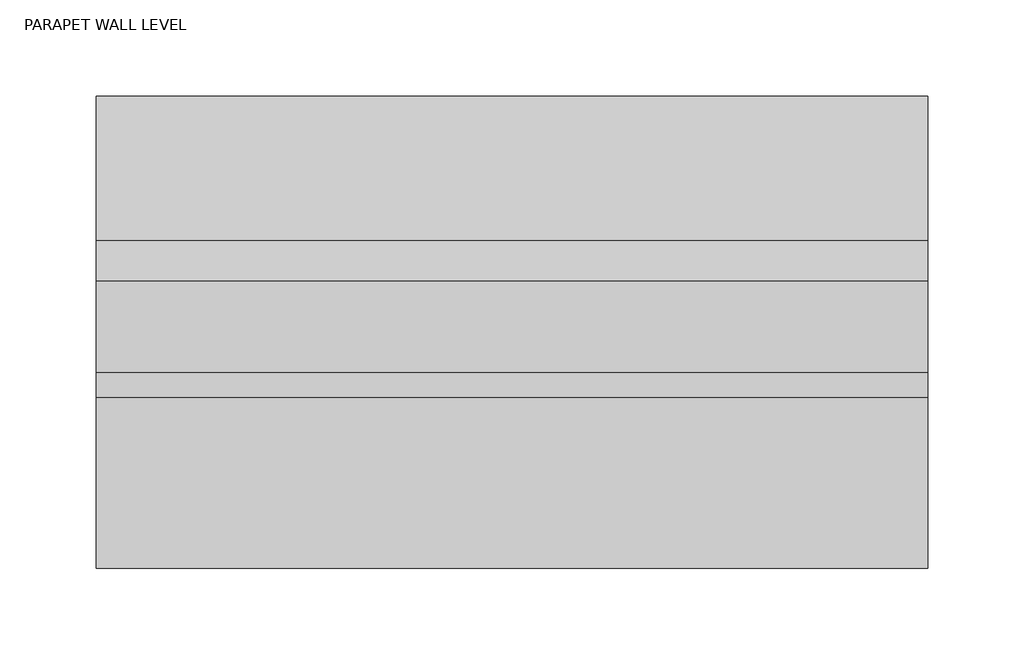
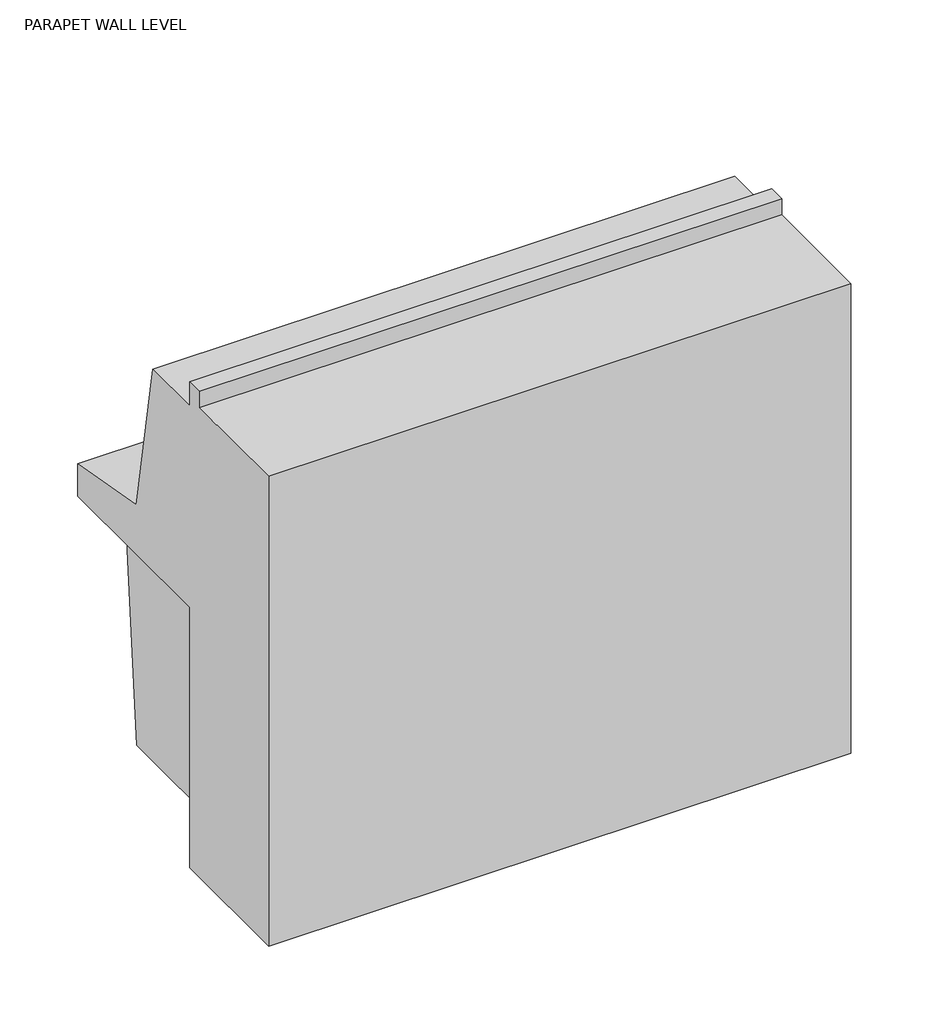
# One storey: 1 light fixture.
"""IFC4 building model written with IfcOpenShell, lengths in millimetres."""

from ifc_helpers import new_model, si_unit, origin, place, context, project, spatial, transform, mapped, element, save
from components import wall_pack_light_exterior_120v_663ef98a

model = new_model("IFC4")

# Units and contexts
model_context = context("Model", 3, world=origin())
ifc_project = project(units=[si_unit("LENGTHUNIT", "METRE", prefix="MILLI")], contexts=[model_context])

# Site, building, storey
site = spatial("IfcSite", under=ifc_project)
building = spatial("IfcBuilding", under=site)
storey = spatial("IfcBuildingStorey", under=building, Name="PARAPET WALL LEVEL", Elevation=9144.0)

# Light fixture
placement = place(None, origin())
wall_pack_light_exterior_120v_shape = wall_pack_light_exterior_120v_663ef98a(model_context)
element("IfcLightFixture", 1, ObjectType="Wall Pack Light - Exterior : 120V", at=placement, inside=storey, context=model_context, shape_type="MappedRepresentation", body=[
    mapped(wall_pack_light_exterior_120v_shape, transform((-17851.5327615, -12241.7027976, 7315.7128848), x_axis=(1.0, 0.0, 0.0), y_axis=(0.0, 1.0, 0.0), z_axis=(0.0, 0.0, 1.0))),
])

save(model, "model.ifc")

# Revit data of these elements
# Type "Wall Pack Light - Exterior : 120V"
#   Assembly Code = "D5020230"
#   Wattage = 300 W
#   built-in parameter 1150110 = 1 (stored number, unit not read)
#   built-in parameter 1114217 = 1 (stored number, unit not read)
#   built-in parameter 1150109 = 1 (stored number, unit not read)
#   built-in parameter 1150113 = 1 (stored number, unit not read)
#   built-in parameter 1150115 = 1 (stored number, unit not read)
#   built-in parameter 1150105 = 1875.72 (stored number, unit not read)
#   Light Source Symbol Size = 2' - 0"
#   built-in parameter 1150112 = 1 (stored number, unit not read)
#   built-in parameter 1150114 = 1 (stored number, unit not read)
#   built-in parameter 1150107 = 4000 (stored number, unit not read)
#   built-in parameter 1150106 = 18.7572 (stored number, unit not read)
#   built-in parameter 1150104 = 7.29939 (stored number, unit not read)
#   Ballast Voltage = 120 V
#   built-in parameter 1114218 = 1 (stored number, unit not read)
#   built-in parameter 1150133 = 10 (stored number, unit not read)
#   Lumens = 23571 lm
#   Mounting Height = 9' - 0"
#   Apparent Load = 70 VA
#   built-in parameter 1150134 = 12
#   built-in parameter 1150137 = 1
#   Color Filter = 16777215
#   Ballast Number of Poles = 1
#   Wall Mount Material = Metal - Paint Finish - Dark Grey, Matte
#   Shade Material = Glass
#   Load Classification = Lighting - Exterior
#   Dimming Lamp Color Temperature Shift = (empty or 0)
#   Default Elevation = 0
# Element 1 (IfcLightFixture, "Wall Pack Light - Exterior : 120V")
#   Mark = "2"
#   Phase Created = New Construction
#   Materials on its faces: "Metal - Paint Finish - Dark Grey, Matte", "Glass"
# Materials
#   "Metal - Paint Finish - Dark Grey, Matte": class "Paint", colour RGB 98 98 98, transparency 0
#   "Glass": class "Glass", colour RGB 0 128 192, transparency 0.75, Description = "Soda Lime Glass", Cost = 0
